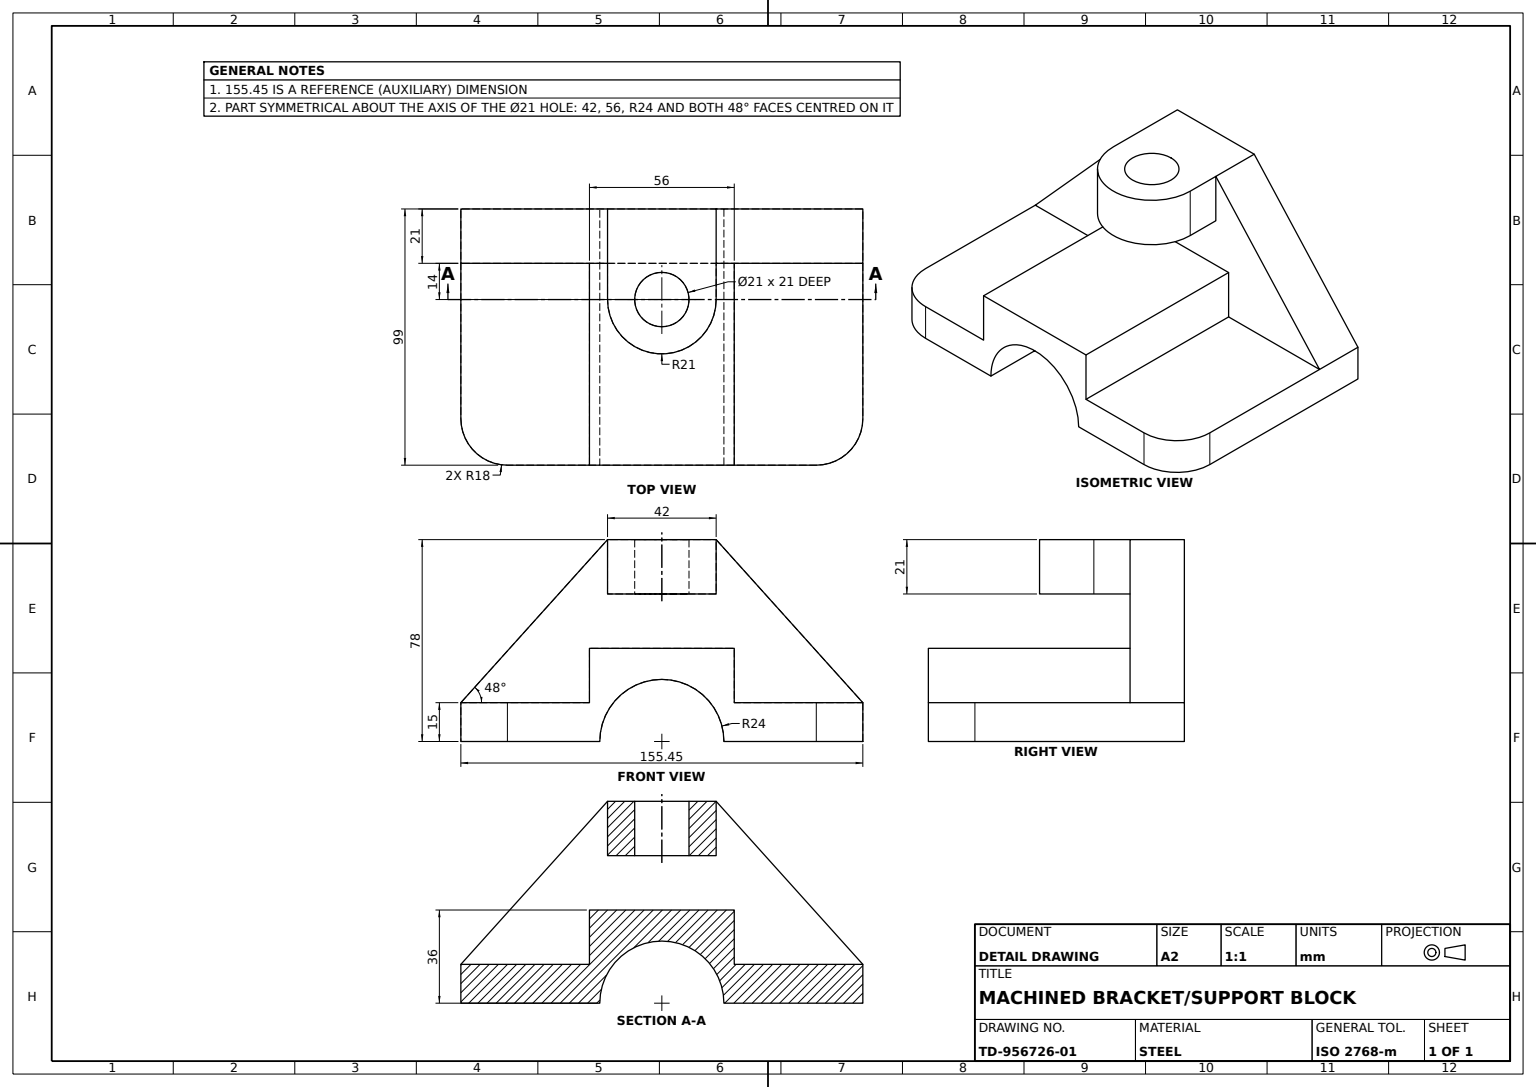
SolidWorks part; units mm, degrees
material "Plain Carbon Steel"
ref_plane "Front Plane" through (0, 0, 0) normal (0, 0, 1) x (1, 0, 0)
ref_plane "Top Plane" through (0, 0, 0) normal (0, 1, 0) x (1, 0, 0)
ref_plane "Right Plane" through (0, 0, 0) normal (1, 0, 0) x (0, 0, -1)
sketch "Base Plate Sketch" plane through (0, 0, 0) normal (0, 1, 0) x (1, 0, 0)
  line L0 (-21, 0) -> (-21, 35)
  line L1 (-21, 35) -> (21, 35)
  line L2 (21, 35) -> (21, 0)
  arc A0 (-21, 0) -> (21, 0) centre (0, 0) ccw
  circle A1 centre (0, 0) radius 10.5
  dimension "D3" = 21
  dimension "D1" = 42
  dimension "D2" = 35
extrude "Base Plate" add sketch "Base Plate Sketch" along normal blind 21
sketch "Angled Web Sketch" plane through (0, 0, -35) normal (0, 0, -1) x (-1, 0, 0)
  line L0 (-77.7255, -42) -> (77.7255, -42) construction
  line L1 (77.7255, -42) -> (77.7255, -57)
  line L2 (77.7255, -57) -> (-77.7255, -57)
  line L3 (-77.7255, -57) -> (-77.7255, -42)
  line L4 (-21, 21) -> (21, 21) construction
  line L5 (-77.7255, -42) -> (-21, 21)
  line L6 (21, 21) -> (77.7255, -42)
  line L7 (-21, 21) -> (21, 21)
  point P2 (0, -57)
  dimension "D1" = 15
  dimension "D2" = 78
  dimension "D3" = 48
extrude "Angled Web 48deg" add sketch "Angled Web Sketch" against normal blind 21
sketch "Upright Block Sketch" plane through (0, 0, -14) normal (0, 0, 1) x (1, 0, 0)
  line L0 (-77.7255, -42) -> (-28, -42)
  line L1 (-28, -42) -> (-28, -21)
  line L2 (-28, -21) -> (28, -21)
  line L3 (28, -21) -> (28, -42)
  line L4 (28, -42) -> (77.7255, -42)
  line L5 (-77.7255, -42) -> (-77.7255, -57)
  line L6 (-77.7255, -57) -> (77.7255, -57)
  line L7 (77.7255, -57) -> (77.7255, -42)
  point P8 (0, -21)
  dimension "D1" = 56
  dimension "D2" = 36
extrude "Upright Block" add sketch "Upright Block Sketch" along normal blind 78
fillet "Corner Fillets R18" radius 18 2 edges at (77.7255, -49.5, 64) (-77.7255, -49.5, 64)
sketch "Half-Round Cut Sketch" plane through (0, 0, 64) normal (0, 0, 1) x (1, 0, 0)
  line L0 (-59.7255, -57) -> (59.7255, -57) construction
  line L1 (-24, -57) -> (24, -57)
  arc A0 (-24, -57) -> (24, -57) centre (0, -57) cw
  dimension "D1" = 24
extrude "Half-Round Cut Ø24" cut sketch "Half-Round Cut Sketch" against normal up to next
